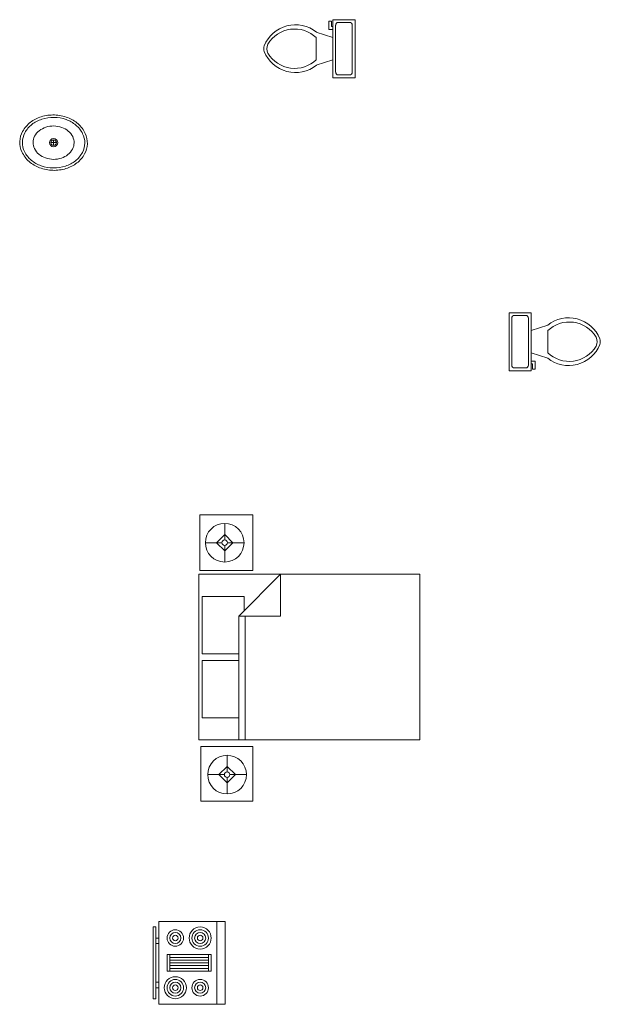
# Model space of a CAD drawing. Units: inches. Extents: x 50 to 2003, y -28 to 675.
# Tile 9 of 10: x 1386 to 1596, y 198 to 554. Entities that reach past the tile are written whole.
import ezdxf

# ---------------------------------------------------------------- set-up
doc = ezdxf.new("R2010")
doc.units = ezdxf.units.IN
for name, color, linetype, lineweight in [('A-EQPM', 8, 'Continuous', 18), ('A-FLOR-FIXT', 9, 'Continuous', 18), ('A-FURN', 8, 'Continuous', 18), ('A-FURN-LITE', 9, 'Continuous', 13)]:
    doc.layers.add(name, color=color, linetype=linetype, lineweight=lineweight)

# ---------------------------------------------------------------- blocks, each defined once
blk = doc.blocks.new('Bed - Queen')
for p, q in [((0, -80.00003), (0, 0)), ((0, 0), (59.99999, 0)), ((59.99999, 0), (59.99999, -80.00003)), ((7.99999, -1.2), (28.79998, -1.2)), ((7.99999, -14.4), (7.99999, -1.2)), ((28.79998, -1.2), (28.79998, -14.4)), ((31.19999, -1.2), (51.99999, -1.2)), ((31.19999, -14.4), (31.19999, -1.2)), ((51.99999, -1.2), (51.99999, -16.4)), ((0, -14.4), (44.8, -14.4)), ((44.8, -16.8), (0, -16.8)), ((59.99999, -29.6), (44.8, -14.4)), ((44.8, -14.4), (44.8, -29.6)), ((51.99999, -16.4), (46.79936, -16.4)), ((44.8, -29.6), (59.99999, -29.6)), ((59.99999, -80.00003), (0, -80.00003))]:
    blk.add_line(p, q)
blk = doc.blocks.new('Lamp - Table')
for p, q in [((0, 7), (0, 1)), ((-1, 0), (-7, 0)), ((0, 3), (-3, 0)), ((-3, 0), (0, -3)), ((3, 0), (0, 3)), ((0, -3), (3, 0)), ((1, 0), (7, 0)), ((0, -1), (0, -7))]:
    blk.add_line(p, q)
for radius in [7, 1]:
    blk.add_circle((0, 0), radius)
blk = doc.blocks.new('Toilet - top')
for p, q in [((9.5, -6), (9.5, -2)), ((-10, -8.5), (-8, -8.5)), ((-10, -9.5), (-10, -8.5)), ((-7, -9.5), (-10, -9.5)), ((-8, -8.5), (-8, -8)), ((-7, -8), (-7, -9.5)), ((-4, -8), (-6, -14)), ((4, -8), (6, -14)), ((4, -14), (-4, -14))]:
    blk.add_line(p, q)
blk.add_lwpolyline([(10.5, -8), (10.5, 0), (-10.5, 0), (-10.5, -8)], close=True)
for points in [[(-9.5, -2), (-9.5, -6)], [(8.5, -1), (-8.5, -1)], [(-8.5, -7), (8.5, -7)]]:
    blk.add_lwpolyline(points)
for centre, radius, start, end in [((-8.62, -1.88), 0.884, 81.8699, 188.1301), ((8.62, -1.88), 0.884, 351.8699, 98.1301), ((-8.62, -6.12), 0.884, 171.8699, 278.1301), ((8.62, -6.12), 0.884, 261.8699, 8.1301), ((3.52, -21.58), 12.17, 141.4691, 247.9714), ((4.2, -21.82), 11.33, 136.3677, 238.9468), ((-3.52, -21.58), 12.17, 292.0284, 38.5307), ((-4.2, -21.82), 11.33, 301.053, 43.6321), ((0, -27.88), 4, 245.7318, 294.2682), ((0, -29), 4, 254.8605, 285.1395)]:
    blk.add_arc(centre, radius, start, end)
blk = doc.blocks.new('Sink - Oval top')
for p, q in [((-1, 0), (1, 0)), ((0, 1), (0, -1))]:
    blk.add_line(p, q)
for points in [[(-12.23, 0.39, 0.117634), (-11.46, -3.36, 0.104469), (-8.88, -6.8, 0.090016), (-5.08, -9.07, 0.08192), (-0.32, -10.02, 0.08192), (4.49, -9.38, 0.090016), (8.42, -7.36, 0.104469), (11.22, -4.09, 0.117634), (12.23, -0.39, 0.117634), (11.46, 3.36, 0.104469), (8.88, 6.8, 0.090016), (5.08, 9.07, 0.08192), (0.32, 10.02, 0.08192), (-4.49, 9.38, 0.090016), (-8.42, 7.36, 0.104469), (-11.22, 4.09, 0.117634)], [(-11.29, 0.16, 0.118622), (-10.52, -3.25, 0.104678), (-8.07, -6.36, 0.089562), (-4.54, -8.37, 0.081185), (-0.13, -9.15, 0.081185), (4.3, -8.49, 0.089562), (7.89, -6.58, 0.104678), (10.42, -3.55, 0.118622), (11.29, -0.16, 0.118622), (10.52, 3.25, 0.104678), (8.07, 6.36, 0.089562), (4.54, 8.37, 0.081185), (0.13, 9.15, 0.081185), (-4.3, 8.49, 0.089562), (-7.89, 6.58, 0.104678), (-10.42, 3.55, 0.118622)], [(-7.42, 0.08, 0.118283), (-6.91, -2.17, 0.104607), (-5.29, -4.21, 0.089718), (-2.97, -5.53, 0.081436), (-0.07, -6.04, 0.081436), (2.84, -5.59, 0.089718), (5.2, -4.33, 0.104607), (6.86, -2.32, 0.118283), (7.42, -0.08, 0.118283), (6.91, 2.17, 0.104607), (5.29, 4.21, 0.089718), (2.97, 5.53, 0.081436), (0.07, 6.04, 0.081436), (-2.84, 5.59, 0.089718), (-5.2, 4.33, 0.104607), (-6.86, 2.32, 0.118283)]]:
    blk.add_lwpolyline(points, format="xyb", close=True)
for radius in [1.5, 1]:
    blk.add_circle((0, 0), radius)
blk = doc.blocks.new('Range-Oven - 30 in top')
for p, q in [((0, -3), (30, -3)), ((12, -6), (18, -6)), ((13, -20), (13, -6)), ((14, -6), (14, -20)), ((15, -20), (15, -6)), ((16, -6), (16, -20)), ((17, -20), (17, -6)), ((18, -20), (12, -20)), ((6, -24), (6, -25)), ((8, -25), (8, -24)), ((22, -25), (22, -24)), ((24, -24), (24, -25))]:
    blk.add_line(p, q)
for points in [[(0, -24), (0, 0), (30, 0), (30, -24)], [(12, -21), (12, -5), (18, -5), (18, -21)], [(2, -26), (2, -25), (28, -25), (28, -26)]]:
    blk.add_lwpolyline(points, close=True)
for centre, radius in [((6, -9), 4), ((6, -9), 3), ((6, -9), 2), ((24, -9), 3), ((24, -9), 2), ((6, -9), 1), ((24, -9), 1), ((24, -18), 4), ((6, -18), 3), ((6, -18), 2), ((6, -18), 1), ((24, -18), 3), ((24, -18), 2), ((24, -18), 1)]:
    blk.add_circle(centre, radius)
blk = doc.blocks.new('NIGHTSTAND-COMPACT')
blk.add_lwpolyline([(0, 19.73), (0, 0), (18.92, 0), (18.92, 19.73)], close=True)
blk = doc.blocks.new('NIGHTSTAND-STANDARD')
blk.add_lwpolyline([(0, 0), (0, 20.13), (19.19, 20.13), (19.19, 0)], close=True)

msp = doc.modelspace()

# ---------------------------------------------------------------- block references
at = {"layer": 'A-EQPM', "rotation": 270}
msp.add_blockref('Range-Oven - 30 in top', (1460.3068, 227.953), dxfattribs=at)
at = {"layer": 'A-FLOR-FIXT'}
for p, rotation in [((1507.3635, 543.9614), 270), ((1563.1337, 437.8733), 89.99999999999999)]:
    msp.add_blockref('Toilet - top', p, dxfattribs=dict(at, rotation=rotation))
msp.add_blockref('Sink - Oval top', (1398.2366, 509.9375), dxfattribs=at)
at = {"layer": 'A-FURN'}
for name, p in [('NIGHTSTAND-STANDARD', (1451.242, 355.0175)), ('NIGHTSTAND-COMPACT', (1451.5085, 271.5474))]:
    msp.add_blockref(name, p, dxfattribs=at)
at = {"layer": 'A-FURN', "rotation": 90}
msp.add_blockref('Bed - Queen', (1450.8483, 293.6639), dxfattribs=at)
at = {"layer": 'A-FURN-LITE', "rotation": 90}
for p in [(1460.1837, 365.0996), (1461.0567, 281.1018)]:
    msp.add_blockref('Lamp - Table', p, dxfattribs=at)

doc.saveas('drawing.dxf')
